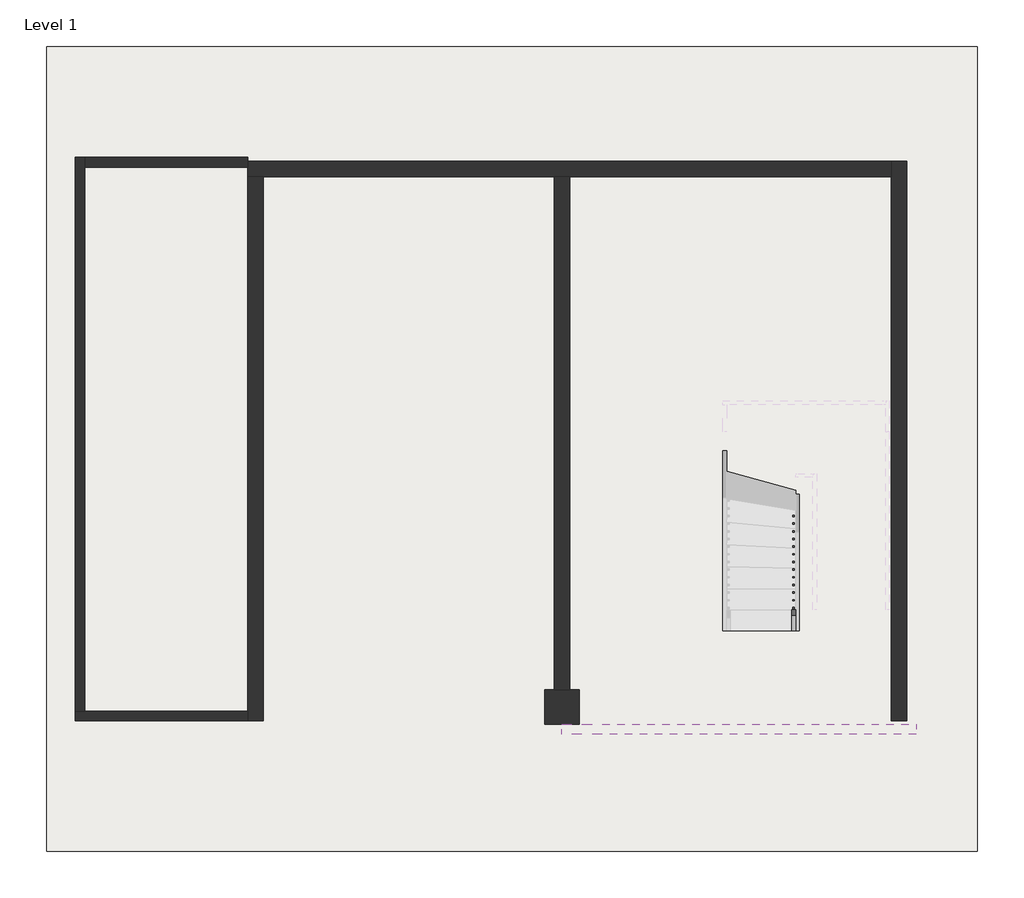
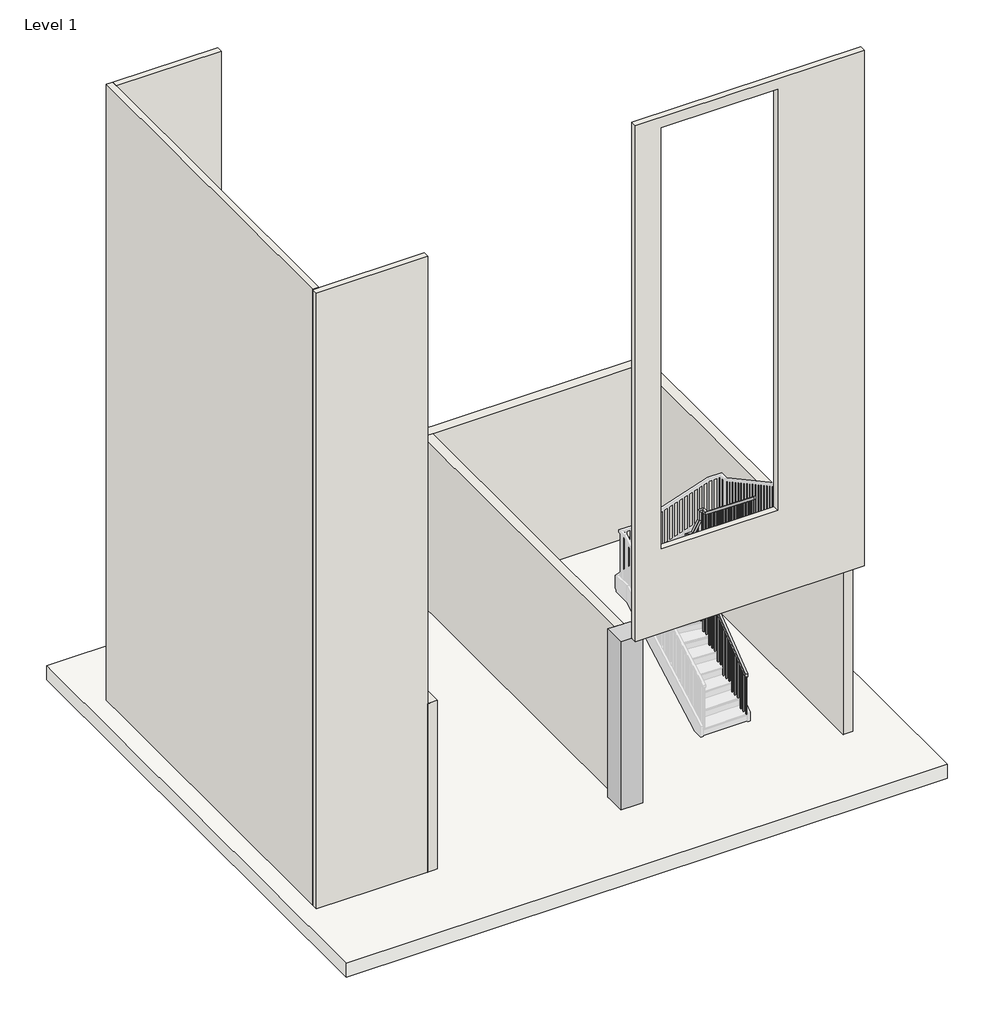
# One storey, part 1 of 2: 8 walls, 1 column, 1 railing, 1 slab.
"""IFC4 building model written with IfcOpenShell, lengths in millimetres."""

from ifc_helpers import new_model, si_unit, frame, origin, origin_with_axes, place, context, project, spatial, polyline, outline, extrude, faceted_brep, element, save

model = new_model("IFC4")

# Units and contexts
model_context = context("Model", 3, world=origin())
ifc_project = project(units=[si_unit("LENGTHUNIT", "METRE", prefix="MILLI")], contexts=[model_context])

# Site, building, storey
site = spatial("IfcSite", under=ifc_project)
building = spatial("IfcBuilding", under=site)
storey = spatial("IfcBuildingStorey", under=building, Name="Level 1", Elevation=0.0)

# Column
placement = place(None, origin())
element("IfcColumn", 1, ObjectType="Rectangular Column : 18\" x 18\"", at=placement, inside=storey, context=model_context, shape_type="Brep", body=[
    faceted_brep([(-10062.032922, 5268.6617654, 3657.6), (-10189.032922, 5268.6617654, 3657.6), (-10392.232922, 5268.6617654, 3657.6), (-10519.232922, 5268.6617654, 3657.6), (-10519.232922, 4811.4617654, 3657.6), (-10062.032922, 4811.4617654, 3657.6), (-10062.032922, 5268.6617654, 0.0), (-10062.032922, 4811.4617654, 0.0), (-10519.232922, 4811.4617654, 0.0), (-10519.232922, 5268.6617654, 0.0), (-10392.232922, 5268.6617654, 0.0), (-10189.032922, 5268.6617654, 0.0)], [[[0, 1, 2, 3, 4, 5]], [[6, 7, 8, 9, 10, 11]], [[3, 2, 1, 0, 6, 11, 10, 9]], [[4, 3, 9, 8]], [[5, 4, 8, 7]], [[0, 5, 7, 6]]]),
])

# Railing
element("IfcRailing", 2, ObjectType="Handrail - Rectangular", at=placement, inside=storey, context=model_context, shape_type="SolidModel", body=[
    faceted_brep([(-7242.632922, 6052.3300735, 1047.0434898), (-7242.632922, 6052.3300735, 982.8664163), (-7191.832922, 6052.3300735, 982.8664163), (-7191.832922, 6052.3300735, 1047.0434898), (-7242.632922, 8062.6617654, 2599.0380287), (-7242.632922, 8113.4617654, 2574.079022), (-7191.832922, 8113.4617654, 2574.079022), (-7191.832922, 8062.6617654, 2599.0380287), (-7242.632922, 8062.6617654, 2805.8347079), (-7242.632922, 8113.4617654, 2755.0347079), (-7191.832922, 8113.4617654, 2755.0347079), (-7191.832922, 8062.6617654, 2805.8347079), (-7242.632922, 8189.6617654, 2805.8347079), (-7242.632922, 8189.6617654, 2755.0347079), (-7191.832922, 8138.8617654, 2755.0347079), (-7191.832922, 8138.8617654, 2805.8347079), (-7115.632922, 8189.6617654, 2805.8347079), (-7086.0984722, 8189.6617654, 2755.0347079), (-7086.0984722, 8138.8617654, 2755.0347079), (-7115.632922, 8138.8617654, 2805.8347079), (-6988.632922, 8189.6617654, 3028.9081493), (-6937.832922, 8189.6617654, 3015.4607435), (-6937.832922, 8138.8617654, 3015.4607435), (-6988.632922, 8138.8617654, 3028.9081493), (-6988.632922, 8189.6617654, 3237.7174934), (-6937.832922, 8189.6617654, 3186.9174934), (-6937.832922, 8138.8617654, 3186.9174934), (-6988.632922, 8138.8617654, 3237.7174934), (-6861.632922, 8189.6617654, 3237.7174934), (-6861.632922, 8189.6617654, 3186.9174934), (-6912.432922, 8138.8617654, 3186.9174934), (-6912.432922, 8138.8617654, 3237.7174934), (-6861.632922, 8062.6617654, 3237.7174934), (-6861.632922, 8044.8554437, 3186.9174934), (-6912.432922, 8044.8554437, 3186.9174934), (-6912.432922, 8062.6617654, 3237.7174934), (-6861.632922, 6331.7300735, 4621.1340886), (-6912.432922, 6331.7300735, 4621.1340886), (-6912.432922, 6331.7300735, 4556.1027004), (-6861.632922, 6331.7300735, 4556.1027004)], [[[0, 1, 2, 3]], [[1, 0, 4, 5]], [[2, 1, 5, 6]], [[3, 2, 6, 7]], [[0, 3, 7, 4]], [[5, 4, 8, 9]], [[6, 5, 9, 10]], [[7, 6, 10, 11]], [[4, 7, 11, 8]], [[9, 8, 12, 13]], [[10, 9, 13, 14]], [[11, 10, 14, 15]], [[8, 11, 15, 12]], [[13, 12, 16, 17]], [[14, 13, 17, 18]], [[15, 14, 18, 19]], [[12, 15, 19, 16]], [[17, 16, 20, 21]], [[18, 17, 21, 22]], [[19, 18, 22, 23]], [[16, 19, 23, 20]], [[21, 20, 24, 25]], [[22, 21, 25, 26]], [[23, 22, 26, 27]], [[20, 23, 27, 24]], [[25, 24, 28, 29]], [[26, 25, 29, 30]], [[27, 26, 30, 31]], [[24, 27, 31, 28]], [[29, 28, 32, 33]], [[30, 29, 33, 34]], [[31, 30, 34, 35]], [[28, 31, 35, 32]], [[36, 37, 38, 39]], [[33, 32, 36, 39]], [[34, 33, 39, 38]], [[35, 34, 38, 37]], [[32, 35, 37, 36]]]),
    extrude(outline(polyline([(6395.7241044, 4504.956601), (6414.7741044, 4489.7312248), (6414.7741044, 3483.4285714), (6395.7241044, 3483.4285714), (6395.7241044, 4504.956601)])), frame((-6896.557922, 0.0, 0.0), z_axis=(1.0, 0.0, 0.0), x_axis=(0.0, 1.0, 0.0)), (0.0, 0.0, 1.0), 19.05),
    extrude(outline(polyline([(6497.3241044, 4423.7545948), (6516.3741044, 4408.5292186), (6516.3741044, 3483.4285714), (6497.3241044, 3483.4285714), (6497.3241044, 4423.7545948)])), frame((-6896.557922, 0.0, 0.0), z_axis=(1.0, 0.0, 0.0), x_axis=(0.0, 1.0, 0.0)), (0.0, 0.0, 1.0), 19.05),
    extrude(outline(polyline([(6598.9241044, 4342.5525885), (6617.9741044, 4327.3272123), (6617.9741044, 3483.4285714), (6598.9241044, 3483.4285714), (6598.9241044, 4342.5525885)])), frame((-6896.557922, 0.0, 0.0), z_axis=(1.0, 0.0, 0.0), x_axis=(0.0, 1.0, 0.0)), (0.0, 0.0, 1.0), 19.05),
    extrude(outline(polyline([(6700.5241044, 4261.3505823), (6719.5741044, 4246.1252061), (6719.5741044, 3309.2571429), (6700.5241044, 3309.2571429), (6700.5241044, 4261.3505823)])), frame((-6896.557922, 0.0, 0.0), z_axis=(1.0, 0.0, 0.0), x_axis=(0.0, 1.0, 0.0)), (0.0, 0.0, 1.0), 19.05),
    extrude(outline(polyline([(6802.1241044, 4180.148576), (6821.1741044, 4164.9231998), (6821.1741044, 3309.2571429), (6802.1241044, 3309.2571429), (6802.1241044, 4180.148576)])), frame((-6896.557922, 0.0, 0.0), z_axis=(1.0, 0.0, 0.0), x_axis=(0.0, 1.0, 0.0)), (0.0, 0.0, 1.0), 19.05),
    extrude(outline(polyline([(6903.7241044, 4098.9465697), (6922.7741044, 4083.7211936), (6922.7741044, 3135.0857143), (6903.7241044, 3135.0857143), (6903.7241044, 4098.9465697)])), frame((-6896.557922, 0.0, 0.0), z_axis=(1.0, 0.0, 0.0), x_axis=(0.0, 1.0, 0.0)), (0.0, 0.0, 1.0), 19.05),
    extrude(outline(polyline([(7005.3241044, 4017.7445635), (7024.3741044, 4002.5191873), (7024.3741044, 3135.0857143), (7005.3241044, 3135.0857143), (7005.3241044, 4017.7445635)])), frame((-6896.557922, 0.0, 0.0), z_axis=(1.0, 0.0, 0.0), x_axis=(0.0, 1.0, 0.0)), (0.0, 0.0, 1.0), 19.05),
    extrude(outline(polyline([(7106.9241044, 3936.5425572), (7125.9741044, 3921.3171811), (7125.9741044, 3135.0857143), (7106.9241044, 3135.0857143), (7106.9241044, 3936.5425572)])), frame((-6896.557922, 0.0, 0.0), z_axis=(1.0, 0.0, 0.0), x_axis=(0.0, 1.0, 0.0)), (0.0, 0.0, 1.0), 19.05),
    extrude(outline(polyline([(7208.5241044, 3855.340551), (7227.5741044, 3840.1151748), (7227.5741044, 2960.9142857), (7208.5241044, 2960.9142857), (7208.5241044, 3855.340551)])), frame((-6896.557922, 0.0, 0.0), z_axis=(1.0, 0.0, 0.0), x_axis=(0.0, 1.0, 0.0)), (0.0, 0.0, 1.0), 19.05),
    extrude(outline(polyline([(7310.1241044, 3774.1385447), (7329.1741044, 3758.9131685), (7329.1741044, 2960.9142857), (7310.1241044, 2960.9142857), (7310.1241044, 3774.1385447)])), frame((-6896.557922, 0.0, 0.0), z_axis=(1.0, 0.0, 0.0), x_axis=(0.0, 1.0, 0.0)), (0.0, 0.0, 1.0), 19.05),
    extrude(outline(polyline([(7411.7241044, 3692.9365385), (7430.7741044, 3677.7111623), (7430.7741044, 2786.7428571), (7411.7241044, 2786.7428571), (7411.7241044, 3692.9365385)])), frame((-6896.557922, 0.0, 0.0), z_axis=(1.0, 0.0, 0.0), x_axis=(0.0, 1.0, 0.0)), (0.0, 0.0, 1.0), 19.05),
    extrude(outline(polyline([(7513.3241044, 3611.7345322), (7532.3741044, 3596.509156), (7532.3741044, 2786.7428571), (7513.3241044, 2786.7428571), (7513.3241044, 3611.7345322)])), frame((-6896.557922, 0.0, 0.0), z_axis=(1.0, 0.0, 0.0), x_axis=(0.0, 1.0, 0.0)), (0.0, 0.0, 1.0), 19.05),
    extrude(outline(polyline([(7614.9241044, 3530.532526), (7633.9741044, 3515.3071498), (7633.9741044, 2786.7428571), (7614.9241044, 2786.7428571), (7614.9241044, 3530.532526)])), frame((-6896.557922, 0.0, 0.0), z_axis=(1.0, 0.0, 0.0), x_axis=(0.0, 1.0, 0.0)), (0.0, 0.0, 1.0), 19.05),
    extrude(outline(polyline([(7716.5241044, 3449.3305197), (7735.5741044, 3434.1051435), (7735.5741044, 2612.5714286), (7716.5241044, 2612.5714286), (7716.5241044, 3449.3305197)])), frame((-6896.557922, 0.0, 0.0), z_axis=(1.0, 0.0, 0.0), x_axis=(0.0, 1.0, 0.0)), (0.0, 0.0, 1.0), 19.05),
    extrude(outline(polyline([(7818.1241044, 3368.1285134), (7837.1741044, 3352.9031373), (7837.1741044, 2612.5714286), (7818.1241044, 2612.5714286), (7818.1241044, 3368.1285134)])), frame((-6896.557922, 0.0, 0.0), z_axis=(1.0, 0.0, 0.0), x_axis=(0.0, 1.0, 0.0)), (0.0, 0.0, 1.0), 19.05),
    extrude(outline(polyline([(7919.7241044, 3286.9265072), (7938.7741044, 3271.701131), (7938.7741044, 2438.4), (7919.7241044, 2438.4), (7919.7241044, 3286.9265072)])), frame((-6896.557922, 0.0, 0.0), z_axis=(1.0, 0.0, 0.0), x_axis=(0.0, 1.0, 0.0)), (0.0, 0.0, 1.0), 19.05),
    extrude(outline(polyline([(8021.3241044, 3205.7245009), (8040.3741044, 3190.4991248), (8040.3741044, 2438.4), (8021.3241044, 2438.4), (8021.3241044, 3205.7245009)])), frame((-6896.557922, 0.0, 0.0), z_axis=(1.0, 0.0, 0.0), x_axis=(0.0, 1.0, 0.0)), (0.0, 0.0, 1.0), 19.05),
    extrude(outline(polyline([(2923.3962905, -6990.2469855), (2889.9352743, -7009.2969855), (1915.8857143, -7009.2969855), (1915.8857143, -6990.2469855), (2923.3962905, -6990.2469855)])), frame((0.0, 8154.7367654, 0.0), z_axis=(0.0, 1.0, 0.0), x_axis=(0.0, 0.0, 1.0)), (0.0, 0.0, 1.0), 19.05),
    extrude(outline(polyline([(2744.9375373, -7091.8469855), (2711.4765211, -7110.8969855), (1915.8857143, -7110.8969855), (1915.8857143, -7091.8469855), (2744.9375373, -7091.8469855)])), frame((0.0, 8154.7367654, 0.0), z_axis=(0.0, 1.0, 0.0), x_axis=(0.0, 0.0, 1.0)), (0.0, 0.0, 1.0), 19.05),
    extrude(outline(polyline([(8074.8050735, 2544.2357006), (8093.8550735, 2558.9424757), (8093.8550735, 1567.5428571), (8074.8050735, 1567.5428571), (8074.8050735, 2544.2357006)])), frame((-7226.757922, 0.0, 0.0), z_axis=(1.0, 0.0, 0.0), x_axis=(0.0, 1.0, 0.0)), (0.0, 0.0, 1.0), 19.05),
    extrude(outline(polyline([(7973.2050735, 2465.799567), (7992.2550735, 2480.5063421), (7992.2550735, 1393.3714286), (7973.2050735, 1393.3714286), (7973.2050735, 2465.799567)])), frame((-7226.757922, 0.0, 0.0), z_axis=(1.0, 0.0, 0.0), x_axis=(0.0, 1.0, 0.0)), (0.0, 0.0, 1.0), 19.05),
    extrude(outline(polyline([(7871.6050735, 2387.3634334), (7890.6550735, 2402.0702085), (7890.6550735, 1219.2), (7871.6050735, 1219.2), (7871.6050735, 2387.3634334)])), frame((-7226.757922, 0.0, 0.0), z_axis=(1.0, 0.0, 0.0), x_axis=(0.0, 1.0, 0.0)), (0.0, 0.0, 1.0), 19.05),
    extrude(outline(polyline([(7770.0050735, 2308.9272998), (7789.0550735, 2323.6340749), (7789.0550735, 1219.2), (7770.0050735, 1219.2), (7770.0050735, 2308.9272998)])), frame((-7226.757922, 0.0, 0.0), z_axis=(1.0, 0.0, 0.0), x_axis=(0.0, 1.0, 0.0)), (0.0, 0.0, 1.0), 19.05),
    extrude(outline(polyline([(7668.4050735, 2230.4911663), (7687.4550735, 2245.1979413), (7687.4550735, 1219.2), (7668.4050735, 1219.2), (7668.4050735, 2230.4911663)])), frame((-7226.757922, 0.0, 0.0), z_axis=(1.0, 0.0, 0.0), x_axis=(0.0, 1.0, 0.0)), (0.0, 0.0, 1.0), 19.05),
    extrude(outline(polyline([(7566.8050735, 2152.0550327), (7585.8550735, 2166.7618077), (7585.8550735, 1045.0285714), (7566.8050735, 1045.0285714), (7566.8050735, 2152.0550327)])), frame((-7226.757922, 0.0, 0.0), z_axis=(1.0, 0.0, 0.0), x_axis=(0.0, 1.0, 0.0)), (0.0, 0.0, 1.0), 19.05),
    extrude(outline(polyline([(7465.2050735, 2073.6188991), (7484.2550735, 2088.3256741), (7484.2550735, 1045.0285714), (7465.2050735, 1045.0285714), (7465.2050735, 2073.6188991)])), frame((-7226.757922, 0.0, 0.0), z_axis=(1.0, 0.0, 0.0), x_axis=(0.0, 1.0, 0.0)), (0.0, 0.0, 1.0), 19.05),
    extrude(outline(polyline([(7363.6050735, 1995.1827655), (7382.6550735, 2009.8895405), (7382.6550735, 870.8571429), (7363.6050735, 870.8571429), (7363.6050735, 1995.1827655)])), frame((-7226.757922, 0.0, 0.0), z_axis=(1.0, 0.0, 0.0), x_axis=(0.0, 1.0, 0.0)), (0.0, 0.0, 1.0), 19.05),
    extrude(outline(polyline([(7262.0050735, 1916.7466319), (7281.0550735, 1931.4534069), (7281.0550735, 870.8571429), (7262.0050735, 870.8571429), (7262.0050735, 1916.7466319)])), frame((-7226.757922, 0.0, 0.0), z_axis=(1.0, 0.0, 0.0), x_axis=(0.0, 1.0, 0.0)), (0.0, 0.0, 1.0), 19.05),
    extrude(outline(polyline([(7160.4050735, 1838.3104983), (7179.4550735, 1853.0172733), (7179.4550735, 870.8571429), (7160.4050735, 870.8571429), (7160.4050735, 1838.3104983)])), frame((-7226.757922, 0.0, 0.0), z_axis=(1.0, 0.0, 0.0), x_axis=(0.0, 1.0, 0.0)), (0.0, 0.0, 1.0), 19.05),
    extrude(outline(polyline([(7058.8050735, 1759.8743647), (7077.8550735, 1774.5811397), (7077.8550735, 696.6857143), (7058.8050735, 696.6857143), (7058.8050735, 1759.8743647)])), frame((-7226.757922, 0.0, 0.0), z_axis=(1.0, 0.0, 0.0), x_axis=(0.0, 1.0, 0.0)), (0.0, 0.0, 1.0), 19.05),
    extrude(outline(polyline([(6957.2050735, 1681.4382311), (6976.2550735, 1696.1450061), (6976.2550735, 696.6857143), (6957.2050735, 696.6857143), (6957.2050735, 1681.4382311)])), frame((-7226.757922, 0.0, 0.0), z_axis=(1.0, 0.0, 0.0), x_axis=(0.0, 1.0, 0.0)), (0.0, 0.0, 1.0), 19.05),
    extrude(outline(polyline([(6855.6050735, 1603.0020975), (6874.6550735, 1617.7088725), (6874.6550735, 522.5142857), (6855.6050735, 522.5142857), (6855.6050735, 1603.0020975)])), frame((-7226.757922, 0.0, 0.0), z_axis=(1.0, 0.0, 0.0), x_axis=(0.0, 1.0, 0.0)), (0.0, 0.0, 1.0), 19.05),
    extrude(outline(polyline([(6754.0050735, 1524.5659639), (6773.0550735, 1539.2727389), (6773.0550735, 522.5142857), (6754.0050735, 522.5142857), (6754.0050735, 1524.5659639)])), frame((-7226.757922, 0.0, 0.0), z_axis=(1.0, 0.0, 0.0), x_axis=(0.0, 1.0, 0.0)), (0.0, 0.0, 1.0), 19.05),
    extrude(outline(polyline([(6652.4050735, 1446.1298303), (6671.4550735, 1460.8366053), (6671.4550735, 522.5142857), (6652.4050735, 522.5142857), (6652.4050735, 1446.1298303)])), frame((-7226.757922, 0.0, 0.0), z_axis=(1.0, 0.0, 0.0), x_axis=(0.0, 1.0, 0.0)), (0.0, 0.0, 1.0), 19.05),
    extrude(outline(polyline([(6550.8050735, 1367.6936967), (6569.8550735, 1382.4004718), (6569.8550735, 348.3428571), (6550.8050735, 348.3428571), (6550.8050735, 1367.6936967)])), frame((-7226.757922, 0.0, 0.0), z_axis=(1.0, 0.0, 0.0), x_axis=(0.0, 1.0, 0.0)), (0.0, 0.0, 1.0), 19.05),
    extrude(outline(polyline([(6449.2050735, 1289.2575631), (6468.2550735, 1303.9643382), (6468.2550735, 348.3428571), (6449.2050735, 348.3428571), (6449.2050735, 1289.2575631)])), frame((-7226.757922, 0.0, 0.0), z_axis=(1.0, 0.0, 0.0), x_axis=(0.0, 1.0, 0.0)), (0.0, 0.0, 1.0), 19.05),
    extrude(outline(polyline([(6347.6050735, 1210.8214295), (6366.6550735, 1225.5282046), (6366.6550735, 348.3428571), (6347.6050735, 348.3428571), (6347.6050735, 1210.8214295)])), frame((-7226.757922, 0.0, 0.0), z_axis=(1.0, 0.0, 0.0), x_axis=(0.0, 1.0, 0.0)), (0.0, 0.0, 1.0), 19.05),
    extrude(outline(polyline([(6246.0050735, 1132.3852959), (6265.0550735, 1147.092071), (6265.0550735, 174.1714286), (6246.0050735, 174.1714286), (6246.0050735, 1132.3852959)])), frame((-7226.757922, 0.0, 0.0), z_axis=(1.0, 0.0, 0.0), x_axis=(0.0, 1.0, 0.0)), (0.0, 0.0, 1.0), 19.05),
    extrude(outline(polyline([(6144.4050735, 1053.9491623), (6163.4550735, 1068.6559374), (6163.4550735, 174.1714286), (6144.4050735, 174.1714286), (6144.4050735, 1053.9491623)])), frame((-7226.757922, 0.0, 0.0), z_axis=(1.0, 0.0, 0.0), x_axis=(0.0, 1.0, 0.0)), (0.0, 0.0, 1.0), 19.05),
    extrude(outline(polyline([(-6896.557922, 8141.9741044), (-6877.507922, 8141.9741044), (-6877.507922, 8122.9241044), (-6896.557922, 8122.9241044), (-6896.557922, 8141.9741044)])), frame((0.0, 0.0, 2264.2285714), z_axis=(0.0, 0.0, 1.0), x_axis=(1.0, 0.0, 0.0)), (0.0, 0.0, 1.0), 922.688922),
    extrude(outline(polyline([(-6896.557922, 8154.7367654), (-6896.557922, 8173.7867654), (-6877.507922, 8173.7867654), (-6877.507922, 8154.7367654), (-6896.557922, 8154.7367654)])), frame((0.0, 0.0, 2264.2285714), z_axis=(0.0, 0.0, 1.0), x_axis=(1.0, 0.0, 0.0)), (0.0, 0.0, 1.0), 922.688922),
    extrude(outline(polyline([(-6911.0332663, 8154.7367654), (-6911.0332663, 8173.7867654), (-6891.9832663, 8173.7867654), (-6891.9832663, 8154.7367654), (-6911.0332663, 8154.7367654)])), frame((0.0, 0.0, 2090.0571429), z_axis=(0.0, 0.0, 1.0), x_axis=(1.0, 0.0, 0.0)), (0.0, 0.0, 1.0), 1096.8603506),
    extrude(outline(polyline([(-7212.4969855, 8154.7367654), (-7212.4969855, 8173.7867654), (-7193.4469855, 8173.7867654), (-7193.4469855, 8154.7367654), (-7212.4969855, 8154.7367654)])), frame((0.0, 0.0, 1741.7142857), z_axis=(0.0, 0.0, 1.0), x_axis=(1.0, 0.0, 0.0)), (0.0, 0.0, 1.0), 1013.3204221),
    extrude(outline(polyline([(-7207.707922, 8154.7367654), (-7226.757922, 8154.7367654), (-7226.757922, 8173.7867654), (-7207.707922, 8173.7867654), (-7207.707922, 8154.7367654)])), frame((0.0, 0.0, 1567.5428571), z_axis=(0.0, 0.0, 1.0), x_axis=(1.0, 0.0, 0.0)), (0.0, 0.0, 1.0), 1187.4918507),
    extrude(outline(polyline([(-7207.707922, 8122.2901259), (-7226.757922, 8122.2901259), (-7226.757922, 8141.3401259), (-7207.707922, 8141.3401259), (-7207.707922, 8122.2901259)])), frame((0.0, 0.0, 1567.5428571), z_axis=(0.0, 0.0, 1.0), x_axis=(1.0, 0.0, 0.0)), (0.0, 0.0, 1.0), 1187.4918507),
    extrude(outline(polyline([(6331.7300735, 4556.1027004), (6350.7800735, 4540.8773242), (6350.7800735, 3483.4285714), (6331.7300735, 3483.4285714), (6331.7300735, 4556.1027004)])), frame((-6896.557922, 0.0, 0.0), z_axis=(1.0, 0.0, 0.0), x_axis=(0.0, 1.0, 0.0)), (0.0, 0.0, 1.0), 19.05),
    extrude(outline(polyline([(6052.3300735, 982.8664163), (6071.3800735, 997.5731913), (6071.3800735, 174.1714286), (6052.3300735, 174.1714286), (6052.3300735, 982.8664163)])), frame((-7226.757922, 0.0, 0.0), z_axis=(1.0, 0.0, 0.0), x_axis=(0.0, 1.0, 0.0)), (0.0, 0.0, 1.0), 19.05),
])

# Slab
element("IfcSlab", 3, ObjectType="Generic - 12\"", at=placement, inside=storey, context=model_context, shape_type="SweptSolid", body=[
    extrude(outline(polyline([(-4779.409907, 13801.2471782), (-4779.409907, 3133.2471782), (-17123.809907, 3133.2471782), (-17123.809907, 13801.2471782), (-4779.409907, 13801.2471782)])), frame((0.0, 0.0, -304.8), z_axis=(0.0, 0.0, 1.0), x_axis=(1.0, 0.0, 0.0)), (0.0, 0.0, 1.0), 304.8),
])

# Walls
element("IfcWall", 4, ObjectType="Generic - 5\"", at=placement, inside=storey, context=model_context, shape_type="SweptSolid", body=[
    extrude(outline(polyline([(3657.6, -5591.632922), (14859.0, -5591.632922), (14859.0, -10290.632922), (3657.6, -10290.632922), (3657.6, -5591.632922)]), holes=[polyline([(14630.4, -7369.632922), (5486.4, -7369.632922), (5486.4, -9757.232922), (14630.4, -9757.232922), (14630.4, -7369.632922)])]), frame((0.0, 4684.4617654, 0.0), z_axis=(0.0, 1.0, 0.0), x_axis=(0.0, 0.0, 1.0)), (0.0, 0.0, 1.0), 127.0),
])
element("IfcWall", 5, ObjectType="Generic - 5\"", at=placement, inside=storey, context=model_context, shape_type="Brep", body=[
    faceted_brep([(-14456.232922, 4989.2617654, 13372.8896509), (-14456.232922, 4989.2617654, 0.0), (-16615.232922, 4989.2617654, 0.0), (-16742.232922, 4989.2617654, 0.0), (-16742.232922, 4989.2617654, 13372.8896509), (-14456.232922, 4862.2617654, 0.0), (-14456.232922, 4862.2617654, 3657.6), (-14456.232922, 4862.2617654, 7315.2), (-14456.232922, 4862.2617654, 10972.8), (-14456.232922, 4862.2617654, 13372.8896509), (-16742.232922, 4862.2617654, 13372.8896509), (-16742.232922, 4862.2617654, 0.0)], [[[0, 1, 2, 3, 4]], [[5, 6, 7, 8, 9, 10, 11]], [[3, 2, 1, 5, 11]], [[0, 4, 10, 9]], [[4, 3, 11, 10]], [[0, 9, 8, 7, 6, 5, 1]]]),
])
element("IfcWall", 6, ObjectType="Generic - 5\"", at=placement, inside=storey, context=model_context, shape_type="Brep", body=[
    faceted_brep([(-16615.232922, 4989.2617654, 0.0), (-16615.232922, 12202.8617654, 0.0), (-16615.232922, 12329.8617654, 0.0), (-16615.232922, 12329.8617654, 13379.5382729), (-16615.232922, 12329.8617654, 13380.5839774), (-16615.232922, 4989.2617654, 13380.5839774), (-16742.232922, 4989.2617654, 0.0), (-16742.232922, 4989.2617654, 13372.8896509), (-16742.232922, 4989.2617654, 13380.5839774), (-16742.232922, 12329.8617654, 13380.5839774), (-16742.232922, 12329.8617654, 0.0)], [[[0, 1, 2, 3, 4, 5]], [[6, 7, 8, 9, 10]], [[2, 1, 0, 6, 10]], [[5, 4, 9, 8]], [[0, 5, 8, 7, 6]], [[4, 3, 2, 10, 9]]]),
])
element("IfcWall", 7, ObjectType="Generic - 5\"", at=placement, inside=storey, context=model_context, shape_type="Brep", body=[
    faceted_brep([(-16615.232922, 12202.8617654, 0.0), (-14456.232922, 12202.8617654, 0.0), (-14456.232922, 12202.8617654, 13379.5382729), (-16615.232922, 12202.8617654, 13379.5382729), (-16615.232922, 12329.8617654, 0.0), (-16615.232922, 12329.8617654, 13379.5382729), (-14456.232922, 12329.8617654, 13379.5382729), (-14456.232922, 12329.8617654, 0.0), (-14456.232922, 12279.0617654, 0.0)], [[[0, 1, 2, 3]], [[4, 5, 6, 7]], [[1, 0, 4, 7, 8]], [[3, 2, 6, 5]], [[0, 3, 5, 4]], [[1, 8, 7, 6, 2]]]),
])
element("IfcWall", 8, ObjectType="Generic - 8\"", at=placement, inside=storey, context=model_context, shape_type="Brep", body=[
    faceted_brep([(-14456.232922, 12075.8617654, 0.0), (-14253.032922, 12075.8617654, 0.0), (-10392.232922, 12075.8617654, 0.0), (-10189.032922, 12075.8617654, 0.0), (-5921.832922, 12075.8617654, 0.0), (-5921.832922, 12075.8617654, 3657.6), (-10189.032922, 12075.8617654, 3657.6), (-10392.232922, 12075.8617654, 3657.6), (-14253.032922, 12075.8617654, 3657.6), (-14435.2593035, 12075.8617654, 3657.6), (-14456.232922, 12075.8617654, 3657.6), (-14456.232922, 12279.0617654, 0.0), (-14456.232922, 12279.0617654, 3657.6), (-14435.2593035, 12279.0617654, 3657.6), (-14253.032922, 12279.0617654, 3657.6), (-5921.832922, 12279.0617654, 3657.6), (-5921.832922, 12279.0617654, 0.0), (-14456.232922, 12202.8617654, 0.0)], [[[0, 1, 2, 3, 4, 5, 6, 7, 8, 9, 10]], [[11, 12, 13, 14, 15, 16]], [[4, 3, 2, 1, 0, 17, 11, 16]], [[5, 4, 16, 15]], [[0, 10, 12, 11, 17]], [[10, 9, 13, 12]], [[9, 8, 7, 6, 5, 15, 14, 13]]]),
])
element("IfcWall", 9, ObjectType="Generic - 8\"", at=placement, inside=storey, context=model_context, shape_type="Brep", body=[
    faceted_brep([(-14253.032922, 4862.2617654, 0.0), (-14253.032922, 12075.8617654, 0.0), (-14253.032922, 12075.8617654, 3657.6), (-14253.032922, 6075.1117654, 3657.6), (-14253.032922, 4865.7935836, 3657.6), (-14253.032922, 4862.2617654, 3657.6), (-14456.232922, 4862.2617654, 0.0), (-14456.232922, 4862.2617654, 3657.6), (-14456.232922, 4865.7935836, 3657.6), (-14456.232922, 6075.1117654, 3657.6), (-14456.232922, 12075.8617654, 3657.6), (-14456.232922, 12075.8617654, 0.0), (-14456.232922, 4989.2617654, 0.0), (-14435.2593035, 12075.8617654, 3657.6), (-14435.2593035, 4865.7935836, 3657.6), (-14435.2593035, 4862.2617654, 3657.6)], [[[0, 1, 2, 3, 4, 5]], [[6, 7, 8, 9, 10, 11, 12]], [[1, 0, 6, 12, 11]], [[4, 3, 2, 13, 14]], [[0, 5, 15, 7, 6]], [[2, 1, 11, 10, 13]], [[13, 10, 9, 8, 14]], [[5, 4, 14, 15]], [[14, 8, 7, 15]]]),
])
element("IfcWall", 10, ObjectType="Generic - 8\"", at=placement, inside=storey, context=model_context, shape_type="Brep", body=[
    faceted_brep([(-5921.832922, 12279.0617654, 0.0), (-5921.832922, 12075.8617654, 0.0), (-5921.832922, 4862.2617654, 0.0), (-5921.832922, 4862.2617654, 3657.6), (-5921.832922, 4865.7935836, 3657.6), (-5921.832922, 12075.8617654, 3657.6), (-5921.832922, 12279.0617654, 3657.6), (-5718.632922, 12279.0617654, 0.0), (-5718.632922, 12279.0617654, 3657.6), (-5718.632922, 4865.7935836, 3657.6), (-5718.632922, 4862.2617654, 3657.6), (-5718.632922, 4862.2617654, 0.0)], [[[0, 1, 2, 3, 4, 5, 6]], [[7, 8, 9, 10, 11]], [[2, 1, 0, 7, 11]], [[3, 2, 11, 10]], [[0, 6, 8, 7]], [[4, 3, 10, 9]], [[6, 5, 4, 9, 8]]]),
])
element("IfcWall", 11, ObjectType="Generic - 8\"", at=placement, inside=storey, context=model_context, shape_type="SweptSolid", body=[
    extrude(outline(polyline([(-10189.032922, 12075.8617654), (-10189.032922, 5268.6617654), (-10392.232922, 5268.6617654), (-10392.232922, 12075.8617654), (-10189.032922, 12075.8617654)])), origin_with_axes(), (0.0, 0.0, 1.0), 3657.6),
])

save(model, "model.ifc")

# Revit data of these elements
# Type "Rectangular Column : 18\" x 18\""
#   Assembly Code = "B1010200"
#   Depth = 1' - 6"
#   Offset Base = 0' - 0"
#   Offset Top = 0' - 0"
#   Width = 1' - 6"
#   Material = none
# Type "Handrail - Rectangular"
#   Assembly Code = "C2010400"
#   built-in parameter 1008612 = 0.0416667 (stored number, unit not read)
#   built-in parameter 1008611 = 0.0416667 (stored number, unit not read)
#   built-in parameter 1008609 = 0.333333 (stored number, unit not read)
#   built-in parameter 1008604 = 0.166667 (stored number, unit not read)
#   built-in parameter 1008603 = 0.166667 (stored number, unit not read)
#   Railing Height = 3' - 0"
#   built-in parameter 1008630 = 2
#   built-in parameter 1008610 = 2
#   built-in parameter 1008618 = Baluster - Square : 3/4"
# Type "Generic - 12\""
#   Assembly Code = "B1010"
#   Function = 0
#   Layers, outside or top first: 1' - 0" no material (function 1)
# Type "Generic - 5\""
#   Assembly Code = "B2010"
#   Layers, outside or top first: 0' - 5" no material (function 1)
# Type "Generic - 8\""
#   Assembly Code = "B2010"
#   Layers, outside or top first: 0' - 8" no material (function 1)
# Element 1 (IfcColumn, "Rectangular Column : 18\" x 18\"")
#   Phase Created = New Construction
#   Materials on its faces: "Default Wall"
# Element 2 (IfcRailing, "Handrail - Rectangular")
#   Phase Created = New Construction
# Element 3 (IfcSlab, "Generic - 12\"")
#   Height Offset From Level = 0' - 0"
#   Phase Created = New Construction
#   Materials on its faces: "Default Floor"
# Element 4 (IfcWall, "Generic - 5\"")
#   Top Offset = 36' - 9"
#   Base Offset = 0' - 0"
#   wall height = 48' - 9"
#   Phase Created = New Construction
#   Base Constraint = Level 1
#   Top Constraint = Level 2
#   Materials on its faces: "Default Wall"
# Element 5 (IfcWall, "Generic - 5\"")
#   Top Offset = -4' - 1.50828"
#   Base Offset = 0' - 0"
#   wall height = 43' - 10.49172"
#   Phase Created = New Construction
#   Base Constraint = Level 1
#   Top Constraint = Level 5
#   Materials on its faces: "Default Wall"
# Element 6 (IfcWall, "Generic - 5\"")
#   Top Offset = -4' - 1.20536"
#   Base Offset = 0' - 0"
#   wall height = 43' - 10.79464"
#   Phase Created = New Construction
#   Base Constraint = Level 1
#   Top Constraint = Level 5
#   Materials on its faces: "Default Wall"
# Element 7 (IfcWall, "Generic - 5\"")
#   Top Offset = -4' - 1.24652"
#   Base Offset = 0' - 0"
#   wall height = 43' - 10.75348"
#   Phase Created = New Construction
#   Base Constraint = Level 1
#   Top Constraint = Level 5
#   Materials on its faces: "Default Wall"
# Elements 8, 9, 10, 11 (IfcWall, "Generic - 8\"")
#   Top Offset = 0' - 0"
#   Base Offset = 0' - 0"
#   Unconnected Height = 12' - 0"
#   wall height = 12' - 0"
#   Phase Created = New Construction
#   Base Constraint = Level 1
#   Materials on its faces: "Default Wall"
# Materials
#   "Default Wall": colour RGB 128 128 128, transparency 0
#   "Default Floor": colour RGB 128 128 128, transparency 0
